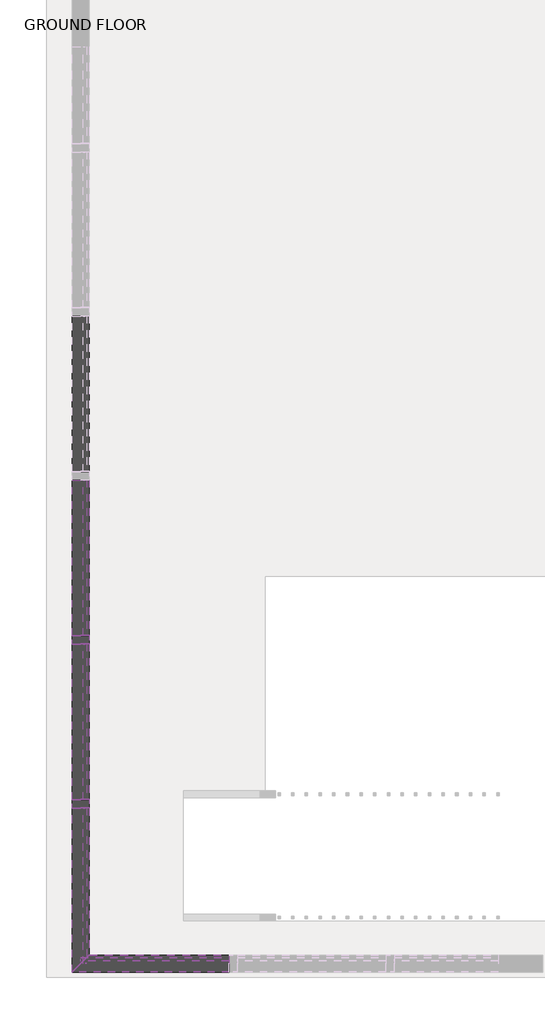
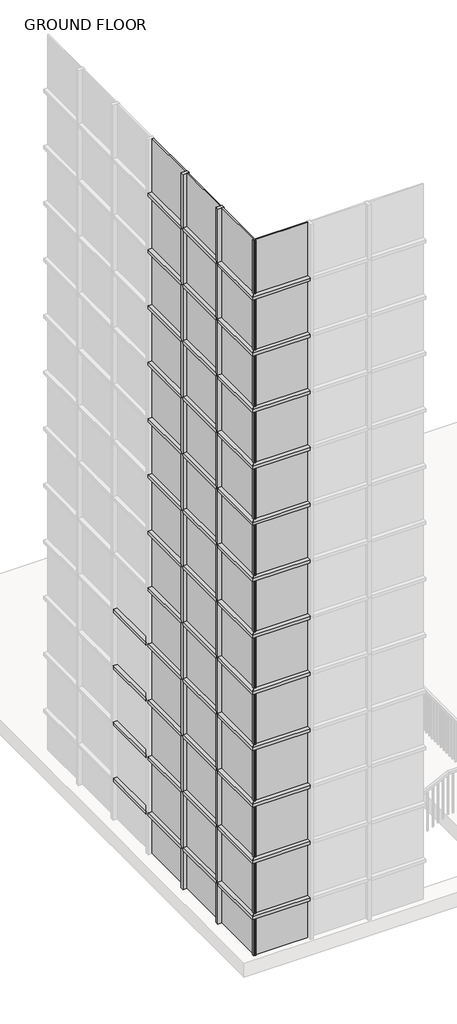
# One storey, part 1 of 16: 78 members, 52 plates.
"""IFC4 building model written with IfcOpenShell, lengths in millimetres."""

from ifc_helpers import new_model, si_unit, origin, place, context, project, spatial, transform, mapped, element, save
from components import member_637f24d3, member_1d29426d, member_b860638c, member_31fee25f, member_49b1bc66, system_panel_glazed_5cba32e5, system_panel_glazed_49652e9e

model = new_model("IFC4")

# Units and contexts
model_context = context("Model", 3, world=origin())
ifc_project = project(units=[si_unit("LENGTHUNIT", "METRE", prefix="MILLI")], contexts=[model_context])

# Site, building, storey
site = spatial("IfcSite", under=ifc_project)
building = spatial("IfcBuilding", under=site)
storey = spatial("IfcBuildingStorey", under=building, Name="GROUND FLOOR", Elevation=0.0)

# Members
placement = place(None, origin())
member_shape = member_637f24d3(model_context)
element("IfcMember", 1, ObjectType="Rectangular Mullion : 2.5\" x 5\" rectangular", at=placement, inside=storey, context=model_context, shape_type="MappedRepresentation", body=[
    mapped(member_shape, transform((-8022.9325224, -5739.2238032, 1168.8884615), x_axis=(0.0, 0.0, 1.0), y_axis=(0.0, -1.0, 0.0), z_axis=(1.0, 0.0, 0.0))),
])
element("IfcMember", 2, ObjectType="Rectangular Mullion : 2.5\" x 5\" rectangular", at=placement, inside=storey, context=model_context, shape_type="MappedRepresentation", body=[
    mapped(member_shape, transform((-8022.9325224, -5739.2238032, 2369.5269231), x_axis=(0.0, 0.0, 1.0), y_axis=(0.0, -1.0, 0.0), z_axis=(1.0, 0.0, 0.0))),
])
element("IfcMember", 3, ObjectType="Rectangular Mullion : 2.5\" x 5\" rectangular", at=placement, inside=storey, context=model_context, shape_type="MappedRepresentation", body=[
    mapped(member_shape, transform((-8022.9325224, -5739.2238032, 3570.1653846), x_axis=(0.0, 0.0, 1.0), y_axis=(0.0, -1.0, 0.0), z_axis=(1.0, 0.0, 0.0))),
])
element("IfcMember", 4, ObjectType="Rectangular Mullion : 2.5\" x 5\" rectangular", at=placement, inside=storey, context=model_context, shape_type="MappedRepresentation", body=[
    mapped(member_shape, transform((-8022.9325224, -5739.2238032, 4770.8038462), x_axis=(0.0, 0.0, 1.0), y_axis=(0.0, -1.0, 0.0), z_axis=(1.0, 0.0, 0.0))),
])
element("IfcMember", 5, ObjectType="Rectangular Mullion : 2.5\" x 5\" rectangular", at=placement, inside=storey, context=model_context, shape_type="MappedRepresentation", body=[
    mapped(member_shape, transform((-8022.9325224, -5739.2238032, 5971.4423077), x_axis=(0.0, 0.0, 1.0), y_axis=(0.0, -1.0, 0.0), z_axis=(1.0, 0.0, 0.0))),
])
element("IfcMember", 6, ObjectType="Rectangular Mullion : 2.5\" x 5\" rectangular", at=placement, inside=storey, context=model_context, shape_type="MappedRepresentation", body=[
    mapped(member_shape, transform((-8022.9325224, -5739.2238032, 7172.0807692), x_axis=(0.0, 0.0, 1.0), y_axis=(0.0, -1.0, 0.0), z_axis=(1.0, 0.0, 0.0))),
])
element("IfcMember", 7, ObjectType="Rectangular Mullion : 2.5\" x 5\" rectangular", at=placement, inside=storey, context=model_context, shape_type="MappedRepresentation", body=[
    mapped(member_shape, transform((-8022.9325224, -5739.2238032, 8372.7192308), x_axis=(0.0, 0.0, 1.0), y_axis=(0.0, -1.0, 0.0), z_axis=(1.0, 0.0, 0.0))),
])
element("IfcMember", 8, ObjectType="Rectangular Mullion : 2.5\" x 5\" rectangular", at=placement, inside=storey, context=model_context, shape_type="MappedRepresentation", body=[
    mapped(member_shape, transform((-8022.9325224, -5739.2238032, 9573.3576923), x_axis=(0.0, 0.0, 1.0), y_axis=(0.0, -1.0, 0.0), z_axis=(1.0, 0.0, 0.0))),
])
element("IfcMember", 9, ObjectType="Rectangular Mullion : 2.5\" x 5\" rectangular", at=placement, inside=storey, context=model_context, shape_type="MappedRepresentation", body=[
    mapped(member_shape, transform((-8022.9325224, -5739.2238032, 10773.9961538), x_axis=(0.0, 0.0, 1.0), y_axis=(0.0, -1.0, 0.0), z_axis=(1.0, 0.0, 0.0))),
])
element("IfcMember", 10, ObjectType="Rectangular Mullion : 2.5\" x 5\" rectangular", at=placement, inside=storey, context=model_context, shape_type="MappedRepresentation", body=[
    mapped(member_shape, transform((-8022.9325224, -5739.2238032, 11974.6346154), x_axis=(0.0, 0.0, 1.0), y_axis=(0.0, -1.0, 0.0), z_axis=(1.0, 0.0, 0.0))),
])
element("IfcMember", 11, ObjectType="Rectangular Mullion : 2.5\" x 5\" rectangular", at=placement, inside=storey, context=model_context, shape_type="MappedRepresentation", body=[
    mapped(member_shape, transform((-8022.9325224, -5739.2238032, 13175.2730769), x_axis=(0.0, 0.0, 1.0), y_axis=(0.0, -1.0, 0.0), z_axis=(1.0, 0.0, 0.0))),
])
element("IfcMember", 12, ObjectType="Rectangular Mullion : 2.5\" x 5\" rectangular", at=placement, inside=storey, context=model_context, shape_type="MappedRepresentation", body=[
    mapped(member_shape, transform((-8022.9325224, -5739.2238032, 14375.9115385), x_axis=(0.0, 0.0, 1.0), y_axis=(0.0, -1.0, 0.0), z_axis=(1.0, 0.0, 0.0))),
])
member_2_shape = member_1d29426d(model_context)
element("IfcMember", 13, ObjectType="Rectangular Mullion : 2.5\" x 5\" rectangular", at=placement, inside=storey, context=model_context, shape_type="MappedRepresentation", body=[
    mapped(member_2_shape, transform((-9124.9017534, -5739.2238032, 1168.8884615), x_axis=(0.0, 0.0, 1.0), y_axis=(-1.0, 0.0, 0.0), z_axis=(0.0, -1.0, 0.0))),
])
element("IfcMember", 14, ObjectType="Rectangular Mullion : 2.5\" x 5\" rectangular", at=placement, inside=storey, context=model_context, shape_type="MappedRepresentation", body=[
    mapped(member_2_shape, transform((-9124.9017534, -5739.2238032, 2369.5269231), x_axis=(0.0, 0.0, 1.0), y_axis=(-1.0, 0.0, 0.0), z_axis=(0.0, -1.0, 0.0))),
])
element("IfcMember", 15, ObjectType="Rectangular Mullion : 2.5\" x 5\" rectangular", at=placement, inside=storey, context=model_context, shape_type="MappedRepresentation", body=[
    mapped(member_2_shape, transform((-9124.9017534, -5739.2238032, 3570.1653846), x_axis=(0.0, 0.0, 1.0), y_axis=(-1.0, 0.0, 0.0), z_axis=(0.0, -1.0, 0.0))),
])
element("IfcMember", 16, ObjectType="Rectangular Mullion : 2.5\" x 5\" rectangular", at=placement, inside=storey, context=model_context, shape_type="MappedRepresentation", body=[
    mapped(member_2_shape, transform((-9124.9017534, -5739.2238032, 4770.8038462), x_axis=(0.0, 0.0, 1.0), y_axis=(-1.0, 0.0, 0.0), z_axis=(0.0, -1.0, 0.0))),
])
element("IfcMember", 17, ObjectType="Rectangular Mullion : 2.5\" x 5\" rectangular", at=placement, inside=storey, context=model_context, shape_type="MappedRepresentation", body=[
    mapped(member_2_shape, transform((-9124.9017534, -5739.2238032, 5971.4423077), x_axis=(0.0, 0.0, 1.0), y_axis=(-1.0, 0.0, 0.0), z_axis=(0.0, -1.0, 0.0))),
])
element("IfcMember", 18, ObjectType="Rectangular Mullion : 2.5\" x 5\" rectangular", at=placement, inside=storey, context=model_context, shape_type="MappedRepresentation", body=[
    mapped(member_2_shape, transform((-9124.9017534, -5739.2238032, 7172.0807692), x_axis=(0.0, 0.0, 1.0), y_axis=(-1.0, 0.0, 0.0), z_axis=(0.0, -1.0, 0.0))),
])
element("IfcMember", 19, ObjectType="Rectangular Mullion : 2.5\" x 5\" rectangular", at=placement, inside=storey, context=model_context, shape_type="MappedRepresentation", body=[
    mapped(member_2_shape, transform((-9124.9017534, -5739.2238032, 8372.7192308), x_axis=(0.0, 0.0, 1.0), y_axis=(-1.0, 0.0, 0.0), z_axis=(0.0, -1.0, 0.0))),
])
element("IfcMember", 20, ObjectType="Rectangular Mullion : 2.5\" x 5\" rectangular", at=placement, inside=storey, context=model_context, shape_type="MappedRepresentation", body=[
    mapped(member_2_shape, transform((-9124.9017534, -5739.2238032, 9573.3576923), x_axis=(0.0, 0.0, 1.0), y_axis=(-1.0, 0.0, 0.0), z_axis=(0.0, -1.0, 0.0))),
])
element("IfcMember", 21, ObjectType="Rectangular Mullion : 2.5\" x 5\" rectangular", at=placement, inside=storey, context=model_context, shape_type="MappedRepresentation", body=[
    mapped(member_2_shape, transform((-9124.9017534, -5739.2238032, 10773.9961538), x_axis=(0.0, 0.0, 1.0), y_axis=(-1.0, 0.0, 0.0), z_axis=(0.0, -1.0, 0.0))),
])
element("IfcMember", 22, ObjectType="Rectangular Mullion : 2.5\" x 5\" rectangular", at=placement, inside=storey, context=model_context, shape_type="MappedRepresentation", body=[
    mapped(member_2_shape, transform((-9124.9017534, -5739.2238032, 11974.6346154), x_axis=(0.0, 0.0, 1.0), y_axis=(-1.0, 0.0, 0.0), z_axis=(0.0, -1.0, 0.0))),
])
element("IfcMember", 23, ObjectType="Rectangular Mullion : 2.5\" x 5\" rectangular", at=placement, inside=storey, context=model_context, shape_type="MappedRepresentation", body=[
    mapped(member_2_shape, transform((-9124.9017534, -5739.2238032, 13175.2730769), x_axis=(0.0, 0.0, 1.0), y_axis=(-1.0, 0.0, 0.0), z_axis=(0.0, -1.0, 0.0))),
])
element("IfcMember", 24, ObjectType="Rectangular Mullion : 2.5\" x 5\" rectangular", at=placement, inside=storey, context=model_context, shape_type="MappedRepresentation", body=[
    mapped(member_2_shape, transform((-9124.9017534, -5739.2238032, 14375.9115385), x_axis=(0.0, 0.0, 1.0), y_axis=(-1.0, 0.0, 0.0), z_axis=(0.0, -1.0, 0.0))),
])
member_3_shape = member_b860638c(model_context)
element("IfcMember", 25, ObjectType="Rectangular Mullion : 2.5\" x 5\" rectangular", at=placement, inside=storey, context=model_context, shape_type="MappedRepresentation", body=[
    mapped(member_3_shape, transform((-9124.9017534, -3336.383803, 0.0), x_axis=(0.0, -1.0, 0.0), y_axis=(-1.0, 0.0, 0.0), z_axis=(0.0, 0.0, -1.0))),
])
element("IfcMember", 26, ObjectType="Rectangular Mullion : 2.5\" x 5\" rectangular", at=placement, inside=storey, context=model_context, shape_type="MappedRepresentation", body=[
    mapped(member_3_shape, transform((-9124.9017534, -4553.678803, 0.0), x_axis=(0.0, -1.0, 0.0), y_axis=(-1.0, 0.0, 0.0), z_axis=(0.0, 0.0, -1.0))),
])
member_4_shape = member_31fee25f(model_context)
element("IfcMember", 27, ObjectType="Rectangular Mullion : 2.5\" x 5\" rectangular", at=placement, inside=storey, context=model_context, shape_type="MappedRepresentation", body=[
    mapped(member_4_shape, transform((-9124.9017534, -3336.383803, 1168.8884615), x_axis=(0.0, -1.0, 0.0), y_axis=(-1.0, 0.0, 0.0), z_axis=(0.0, 0.0, -1.0))),
])
element("IfcMember", 28, ObjectType="Rectangular Mullion : 2.5\" x 5\" rectangular", at=placement, inside=storey, context=model_context, shape_type="MappedRepresentation", body=[
    mapped(member_4_shape, transform((-9124.9017534, -4553.678803, 1168.8884615), x_axis=(0.0, -1.0, 0.0), y_axis=(-1.0, 0.0, 0.0), z_axis=(0.0, 0.0, -1.0))),
])
element("IfcMember", 29, ObjectType="Rectangular Mullion : 2.5\" x 5\" rectangular", at=placement, inside=storey, context=model_context, shape_type="MappedRepresentation", body=[
    mapped(member_4_shape, transform((-9124.9017534, -3336.383803, 2369.5269231), x_axis=(0.0, -1.0, 0.0), y_axis=(-1.0, 0.0, 0.0), z_axis=(0.0, 0.0, -1.0))),
])
element("IfcMember", 30, ObjectType="Rectangular Mullion : 2.5\" x 5\" rectangular", at=placement, inside=storey, context=model_context, shape_type="MappedRepresentation", body=[
    mapped(member_4_shape, transform((-9124.9017534, -4553.678803, 2369.5269231), x_axis=(0.0, -1.0, 0.0), y_axis=(-1.0, 0.0, 0.0), z_axis=(0.0, 0.0, -1.0))),
])
element("IfcMember", 31, ObjectType="Rectangular Mullion : 2.5\" x 5\" rectangular", at=placement, inside=storey, context=model_context, shape_type="MappedRepresentation", body=[
    mapped(member_4_shape, transform((-9124.9017534, -3336.383803, 3570.1653846), x_axis=(0.0, -1.0, 0.0), y_axis=(-1.0, 0.0, 0.0), z_axis=(0.0, 0.0, -1.0))),
])
element("IfcMember", 32, ObjectType="Rectangular Mullion : 2.5\" x 5\" rectangular", at=placement, inside=storey, context=model_context, shape_type="MappedRepresentation", body=[
    mapped(member_4_shape, transform((-9124.9017534, -4553.678803, 3570.1653846), x_axis=(0.0, -1.0, 0.0), y_axis=(-1.0, 0.0, 0.0), z_axis=(0.0, 0.0, -1.0))),
])
element("IfcMember", 33, ObjectType="Rectangular Mullion : 2.5\" x 5\" rectangular", at=placement, inside=storey, context=model_context, shape_type="MappedRepresentation", body=[
    mapped(member_4_shape, transform((-9124.9017534, -3336.383803, 4770.8038462), x_axis=(0.0, -1.0, 0.0), y_axis=(-1.0, 0.0, 0.0), z_axis=(0.0, 0.0, -1.0))),
])
element("IfcMember", 34, ObjectType="Rectangular Mullion : 2.5\" x 5\" rectangular", at=placement, inside=storey, context=model_context, shape_type="MappedRepresentation", body=[
    mapped(member_4_shape, transform((-9124.9017534, -4553.678803, 4770.8038462), x_axis=(0.0, -1.0, 0.0), y_axis=(-1.0, 0.0, 0.0), z_axis=(0.0, 0.0, -1.0))),
])
element("IfcMember", 35, ObjectType="Rectangular Mullion : 2.5\" x 5\" rectangular", at=placement, inside=storey, context=model_context, shape_type="MappedRepresentation", body=[
    mapped(member_4_shape, transform((-9124.9017534, -3336.383803, 5971.4423077), x_axis=(0.0, -1.0, 0.0), y_axis=(-1.0, 0.0, 0.0), z_axis=(0.0, 0.0, -1.0))),
])
element("IfcMember", 36, ObjectType="Rectangular Mullion : 2.5\" x 5\" rectangular", at=placement, inside=storey, context=model_context, shape_type="MappedRepresentation", body=[
    mapped(member_4_shape, transform((-9124.9017534, -4553.678803, 5971.4423077), x_axis=(0.0, -1.0, 0.0), y_axis=(-1.0, 0.0, 0.0), z_axis=(0.0, 0.0, -1.0))),
])
element("IfcMember", 37, ObjectType="Rectangular Mullion : 2.5\" x 5\" rectangular", at=placement, inside=storey, context=model_context, shape_type="MappedRepresentation", body=[
    mapped(member_4_shape, transform((-9124.9017534, -3336.383803, 7172.0807692), x_axis=(0.0, -1.0, 0.0), y_axis=(-1.0, 0.0, 0.0), z_axis=(0.0, 0.0, -1.0))),
])
element("IfcMember", 38, ObjectType="Rectangular Mullion : 2.5\" x 5\" rectangular", at=placement, inside=storey, context=model_context, shape_type="MappedRepresentation", body=[
    mapped(member_4_shape, transform((-9124.9017534, -4553.678803, 7172.0807692), x_axis=(0.0, -1.0, 0.0), y_axis=(-1.0, 0.0, 0.0), z_axis=(0.0, 0.0, -1.0))),
])
element("IfcMember", 39, ObjectType="Rectangular Mullion : 2.5\" x 5\" rectangular", at=placement, inside=storey, context=model_context, shape_type="MappedRepresentation", body=[
    mapped(member_4_shape, transform((-9124.9017534, -3336.383803, 8372.7192308), x_axis=(0.0, -1.0, 0.0), y_axis=(-1.0, 0.0, 0.0), z_axis=(0.0, 0.0, -1.0))),
])
element("IfcMember", 40, ObjectType="Rectangular Mullion : 2.5\" x 5\" rectangular", at=placement, inside=storey, context=model_context, shape_type="MappedRepresentation", body=[
    mapped(member_4_shape, transform((-9124.9017534, -4553.678803, 8372.7192308), x_axis=(0.0, -1.0, 0.0), y_axis=(-1.0, 0.0, 0.0), z_axis=(0.0, 0.0, -1.0))),
])
element("IfcMember", 41, ObjectType="Rectangular Mullion : 2.5\" x 5\" rectangular", at=placement, inside=storey, context=model_context, shape_type="MappedRepresentation", body=[
    mapped(member_4_shape, transform((-9124.9017534, -3336.383803, 9573.3576923), x_axis=(0.0, -1.0, 0.0), y_axis=(-1.0, 0.0, 0.0), z_axis=(0.0, 0.0, -1.0))),
])
element("IfcMember", 42, ObjectType="Rectangular Mullion : 2.5\" x 5\" rectangular", at=placement, inside=storey, context=model_context, shape_type="MappedRepresentation", body=[
    mapped(member_4_shape, transform((-9124.9017534, -4553.678803, 9573.3576923), x_axis=(0.0, -1.0, 0.0), y_axis=(-1.0, 0.0, 0.0), z_axis=(0.0, 0.0, -1.0))),
])
element("IfcMember", 43, ObjectType="Rectangular Mullion : 2.5\" x 5\" rectangular", at=placement, inside=storey, context=model_context, shape_type="MappedRepresentation", body=[
    mapped(member_4_shape, transform((-9124.9017534, -3336.383803, 10773.9961538), x_axis=(0.0, -1.0, 0.0), y_axis=(-1.0, 0.0, 0.0), z_axis=(0.0, 0.0, -1.0))),
])
element("IfcMember", 44, ObjectType="Rectangular Mullion : 2.5\" x 5\" rectangular", at=placement, inside=storey, context=model_context, shape_type="MappedRepresentation", body=[
    mapped(member_4_shape, transform((-9124.9017534, -4553.678803, 10773.9961538), x_axis=(0.0, -1.0, 0.0), y_axis=(-1.0, 0.0, 0.0), z_axis=(0.0, 0.0, -1.0))),
])
element("IfcMember", 45, ObjectType="Rectangular Mullion : 2.5\" x 5\" rectangular", at=placement, inside=storey, context=model_context, shape_type="MappedRepresentation", body=[
    mapped(member_4_shape, transform((-9124.9017534, -3336.383803, 11974.6346154), x_axis=(0.0, -1.0, 0.0), y_axis=(-1.0, 0.0, 0.0), z_axis=(0.0, 0.0, -1.0))),
])
element("IfcMember", 46, ObjectType="Rectangular Mullion : 2.5\" x 5\" rectangular", at=placement, inside=storey, context=model_context, shape_type="MappedRepresentation", body=[
    mapped(member_4_shape, transform((-9124.9017534, -4553.678803, 11974.6346154), x_axis=(0.0, -1.0, 0.0), y_axis=(-1.0, 0.0, 0.0), z_axis=(0.0, 0.0, -1.0))),
])
element("IfcMember", 47, ObjectType="Rectangular Mullion : 2.5\" x 5\" rectangular", at=placement, inside=storey, context=model_context, shape_type="MappedRepresentation", body=[
    mapped(member_4_shape, transform((-9124.9017534, -3336.383803, 13175.2730769), x_axis=(0.0, -1.0, 0.0), y_axis=(-1.0, 0.0, 0.0), z_axis=(0.0, 0.0, -1.0))),
])
element("IfcMember", 48, ObjectType="Rectangular Mullion : 2.5\" x 5\" rectangular", at=placement, inside=storey, context=model_context, shape_type="MappedRepresentation", body=[
    mapped(member_4_shape, transform((-9124.9017534, -4553.678803, 13175.2730769), x_axis=(0.0, -1.0, 0.0), y_axis=(-1.0, 0.0, 0.0), z_axis=(0.0, 0.0, -1.0))),
])
element("IfcMember", 49, ObjectType="Rectangular Mullion : 2.5\" x 5\" rectangular", at=placement, inside=storey, context=model_context, shape_type="MappedRepresentation", body=[
    mapped(member_3_shape, transform((-9124.9017534, -3336.383803, 14375.9115385), x_axis=(0.0, -1.0, 0.0), y_axis=(-1.0, 0.0, 0.0), z_axis=(0.0, 0.0, -1.0))),
])
element("IfcMember", 50, ObjectType="Rectangular Mullion : 2.5\" x 5\" rectangular", at=placement, inside=storey, context=model_context, shape_type="MappedRepresentation", body=[
    mapped(member_3_shape, transform((-9124.9017534, -4553.678803, 14375.9115385), x_axis=(0.0, -1.0, 0.0), y_axis=(-1.0, 0.0, 0.0), z_axis=(0.0, 0.0, -1.0))),
])
member_5_shape = member_49b1bc66(model_context)
element("IfcMember", 51, ObjectType="Rectangular Mullion : 2.5\" x 5\" rectangular", at=placement, inside=storey, context=model_context, shape_type="MappedRepresentation", body=[
    mapped(member_5_shape, transform((-9124.9017534, -2087.3388031, 1168.8884615), x_axis=(0.0, 0.0, 1.0), y_axis=(-1.0, 0.0, 0.0), z_axis=(0.0, -1.0, 0.0))),
])
element("IfcMember", 52, ObjectType="Rectangular Mullion : 2.5\" x 5\" rectangular", at=placement, inside=storey, context=model_context, shape_type="MappedRepresentation", body=[
    mapped(member_5_shape, transform((-9124.9017534, -3304.633803, 1168.8884615), x_axis=(0.0, 0.0, 1.0), y_axis=(-1.0, 0.0, 0.0), z_axis=(0.0, -1.0, 0.0))),
])
element("IfcMember", 53, ObjectType="Rectangular Mullion : 2.5\" x 5\" rectangular", at=placement, inside=storey, context=model_context, shape_type="MappedRepresentation", body=[
    mapped(member_5_shape, transform((-9124.9017534, -4521.928803, 1168.8884615), x_axis=(0.0, 0.0, 1.0), y_axis=(-1.0, 0.0, 0.0), z_axis=(0.0, -1.0, 0.0))),
])
element("IfcMember", 54, ObjectType="Rectangular Mullion : 2.5\" x 5\" rectangular", at=placement, inside=storey, context=model_context, shape_type="MappedRepresentation", body=[
    mapped(member_5_shape, transform((-9124.9017534, -2087.3388031, 2369.5269231), x_axis=(0.0, 0.0, 1.0), y_axis=(-1.0, 0.0, 0.0), z_axis=(0.0, -1.0, 0.0))),
])
element("IfcMember", 55, ObjectType="Rectangular Mullion : 2.5\" x 5\" rectangular", at=placement, inside=storey, context=model_context, shape_type="MappedRepresentation", body=[
    mapped(member_5_shape, transform((-9124.9017534, -3304.633803, 2369.5269231), x_axis=(0.0, 0.0, 1.0), y_axis=(-1.0, 0.0, 0.0), z_axis=(0.0, -1.0, 0.0))),
])
element("IfcMember", 56, ObjectType="Rectangular Mullion : 2.5\" x 5\" rectangular", at=placement, inside=storey, context=model_context, shape_type="MappedRepresentation", body=[
    mapped(member_5_shape, transform((-9124.9017534, -4521.928803, 2369.5269231), x_axis=(0.0, 0.0, 1.0), y_axis=(-1.0, 0.0, 0.0), z_axis=(0.0, -1.0, 0.0))),
])
element("IfcMember", 57, ObjectType="Rectangular Mullion : 2.5\" x 5\" rectangular", at=placement, inside=storey, context=model_context, shape_type="MappedRepresentation", body=[
    mapped(member_5_shape, transform((-9124.9017534, -2087.3388031, 3570.1653846), x_axis=(0.0, 0.0, 1.0), y_axis=(-1.0, 0.0, 0.0), z_axis=(0.0, -1.0, 0.0))),
])
element("IfcMember", 58, ObjectType="Rectangular Mullion : 2.5\" x 5\" rectangular", at=placement, inside=storey, context=model_context, shape_type="MappedRepresentation", body=[
    mapped(member_5_shape, transform((-9124.9017534, -3304.633803, 3570.1653846), x_axis=(0.0, 0.0, 1.0), y_axis=(-1.0, 0.0, 0.0), z_axis=(0.0, -1.0, 0.0))),
])
element("IfcMember", 59, ObjectType="Rectangular Mullion : 2.5\" x 5\" rectangular", at=placement, inside=storey, context=model_context, shape_type="MappedRepresentation", body=[
    mapped(member_5_shape, transform((-9124.9017534, -4521.928803, 3570.1653846), x_axis=(0.0, 0.0, 1.0), y_axis=(-1.0, 0.0, 0.0), z_axis=(0.0, -1.0, 0.0))),
])
element("IfcMember", 60, ObjectType="Rectangular Mullion : 2.5\" x 5\" rectangular", at=placement, inside=storey, context=model_context, shape_type="MappedRepresentation", body=[
    mapped(member_5_shape, transform((-9124.9017534, -2087.3388031, 4770.8038462), x_axis=(0.0, 0.0, 1.0), y_axis=(-1.0, 0.0, 0.0), z_axis=(0.0, -1.0, 0.0))),
])
element("IfcMember", 61, ObjectType="Rectangular Mullion : 2.5\" x 5\" rectangular", at=placement, inside=storey, context=model_context, shape_type="MappedRepresentation", body=[
    mapped(member_5_shape, transform((-9124.9017534, -3304.633803, 4770.8038462), x_axis=(0.0, 0.0, 1.0), y_axis=(-1.0, 0.0, 0.0), z_axis=(0.0, -1.0, 0.0))),
])
element("IfcMember", 62, ObjectType="Rectangular Mullion : 2.5\" x 5\" rectangular", at=placement, inside=storey, context=model_context, shape_type="MappedRepresentation", body=[
    mapped(member_5_shape, transform((-9124.9017534, -4521.928803, 4770.8038462), x_axis=(0.0, 0.0, 1.0), y_axis=(-1.0, 0.0, 0.0), z_axis=(0.0, -1.0, 0.0))),
])
element("IfcMember", 63, ObjectType="Rectangular Mullion : 2.5\" x 5\" rectangular", at=placement, inside=storey, context=model_context, shape_type="MappedRepresentation", body=[
    mapped(member_5_shape, transform((-9124.9017534, -3304.633803, 5971.4423077), x_axis=(0.0, 0.0, 1.0), y_axis=(-1.0, 0.0, 0.0), z_axis=(0.0, -1.0, 0.0))),
])
element("IfcMember", 64, ObjectType="Rectangular Mullion : 2.5\" x 5\" rectangular", at=placement, inside=storey, context=model_context, shape_type="MappedRepresentation", body=[
    mapped(member_5_shape, transform((-9124.9017534, -4521.928803, 5971.4423077), x_axis=(0.0, 0.0, 1.0), y_axis=(-1.0, 0.0, 0.0), z_axis=(0.0, -1.0, 0.0))),
])
element("IfcMember", 65, ObjectType="Rectangular Mullion : 2.5\" x 5\" rectangular", at=placement, inside=storey, context=model_context, shape_type="MappedRepresentation", body=[
    mapped(member_5_shape, transform((-9124.9017534, -3304.633803, 7172.0807692), x_axis=(0.0, 0.0, 1.0), y_axis=(-1.0, 0.0, 0.0), z_axis=(0.0, -1.0, 0.0))),
])
element("IfcMember", 66, ObjectType="Rectangular Mullion : 2.5\" x 5\" rectangular", at=placement, inside=storey, context=model_context, shape_type="MappedRepresentation", body=[
    mapped(member_5_shape, transform((-9124.9017534, -4521.928803, 7172.0807692), x_axis=(0.0, 0.0, 1.0), y_axis=(-1.0, 0.0, 0.0), z_axis=(0.0, -1.0, 0.0))),
])
element("IfcMember", 67, ObjectType="Rectangular Mullion : 2.5\" x 5\" rectangular", at=placement, inside=storey, context=model_context, shape_type="MappedRepresentation", body=[
    mapped(member_5_shape, transform((-9124.9017534, -3304.633803, 8372.7192308), x_axis=(0.0, 0.0, 1.0), y_axis=(-1.0, 0.0, 0.0), z_axis=(0.0, -1.0, 0.0))),
])
element("IfcMember", 68, ObjectType="Rectangular Mullion : 2.5\" x 5\" rectangular", at=placement, inside=storey, context=model_context, shape_type="MappedRepresentation", body=[
    mapped(member_5_shape, transform((-9124.9017534, -4521.928803, 8372.7192308), x_axis=(0.0, 0.0, 1.0), y_axis=(-1.0, 0.0, 0.0), z_axis=(0.0, -1.0, 0.0))),
])
element("IfcMember", 69, ObjectType="Rectangular Mullion : 2.5\" x 5\" rectangular", at=placement, inside=storey, context=model_context, shape_type="MappedRepresentation", body=[
    mapped(member_5_shape, transform((-9124.9017534, -3304.633803, 9573.3576923), x_axis=(0.0, 0.0, 1.0), y_axis=(-1.0, 0.0, 0.0), z_axis=(0.0, -1.0, 0.0))),
])
element("IfcMember", 70, ObjectType="Rectangular Mullion : 2.5\" x 5\" rectangular", at=placement, inside=storey, context=model_context, shape_type="MappedRepresentation", body=[
    mapped(member_5_shape, transform((-9124.9017534, -4521.928803, 9573.3576923), x_axis=(0.0, 0.0, 1.0), y_axis=(-1.0, 0.0, 0.0), z_axis=(0.0, -1.0, 0.0))),
])
element("IfcMember", 71, ObjectType="Rectangular Mullion : 2.5\" x 5\" rectangular", at=placement, inside=storey, context=model_context, shape_type="MappedRepresentation", body=[
    mapped(member_5_shape, transform((-9124.9017534, -3304.633803, 10773.9961538), x_axis=(0.0, 0.0, 1.0), y_axis=(-1.0, 0.0, 0.0), z_axis=(0.0, -1.0, 0.0))),
])
element("IfcMember", 72, ObjectType="Rectangular Mullion : 2.5\" x 5\" rectangular", at=placement, inside=storey, context=model_context, shape_type="MappedRepresentation", body=[
    mapped(member_5_shape, transform((-9124.9017534, -4521.928803, 10773.9961538), x_axis=(0.0, 0.0, 1.0), y_axis=(-1.0, 0.0, 0.0), z_axis=(0.0, -1.0, 0.0))),
])
element("IfcMember", 73, ObjectType="Rectangular Mullion : 2.5\" x 5\" rectangular", at=placement, inside=storey, context=model_context, shape_type="MappedRepresentation", body=[
    mapped(member_5_shape, transform((-9124.9017534, -3304.633803, 11974.6346154), x_axis=(0.0, 0.0, 1.0), y_axis=(-1.0, 0.0, 0.0), z_axis=(0.0, -1.0, 0.0))),
])
element("IfcMember", 74, ObjectType="Rectangular Mullion : 2.5\" x 5\" rectangular", at=placement, inside=storey, context=model_context, shape_type="MappedRepresentation", body=[
    mapped(member_5_shape, transform((-9124.9017534, -4521.928803, 11974.6346154), x_axis=(0.0, 0.0, 1.0), y_axis=(-1.0, 0.0, 0.0), z_axis=(0.0, -1.0, 0.0))),
])
element("IfcMember", 75, ObjectType="Rectangular Mullion : 2.5\" x 5\" rectangular", at=placement, inside=storey, context=model_context, shape_type="MappedRepresentation", body=[
    mapped(member_5_shape, transform((-9124.9017534, -3304.633803, 13175.2730769), x_axis=(0.0, 0.0, 1.0), y_axis=(-1.0, 0.0, 0.0), z_axis=(0.0, -1.0, 0.0))),
])
element("IfcMember", 76, ObjectType="Rectangular Mullion : 2.5\" x 5\" rectangular", at=placement, inside=storey, context=model_context, shape_type="MappedRepresentation", body=[
    mapped(member_5_shape, transform((-9124.9017534, -4521.928803, 13175.2730769), x_axis=(0.0, 0.0, 1.0), y_axis=(-1.0, 0.0, 0.0), z_axis=(0.0, -1.0, 0.0))),
])
element("IfcMember", 77, ObjectType="Rectangular Mullion : 2.5\" x 5\" rectangular", at=placement, inside=storey, context=model_context, shape_type="MappedRepresentation", body=[
    mapped(member_5_shape, transform((-9124.9017534, -3304.633803, 14375.9115385), x_axis=(0.0, 0.0, 1.0), y_axis=(-1.0, 0.0, 0.0), z_axis=(0.0, -1.0, 0.0))),
])
element("IfcMember", 78, ObjectType="Rectangular Mullion : 2.5\" x 5\" rectangular", at=placement, inside=storey, context=model_context, shape_type="MappedRepresentation", body=[
    mapped(member_5_shape, transform((-9124.9017534, -4521.928803, 14375.9115385), x_axis=(0.0, 0.0, 1.0), y_axis=(-1.0, 0.0, 0.0), z_axis=(0.0, -1.0, 0.0))),
])

# Plates
system_panel_glazed_shape = system_panel_glazed_5cba32e5(model_context)
element("IfcPlate", 79, ObjectType="System Panel : Glazed", at=placement, inside=storey, context=model_context, shape_type="MappedRepresentation", body=[
    mapped(system_panel_glazed_shape, transform((-8573.9171379, -5739.2238032, 0.0), x_axis=(1.0, 0.0, 0.0), y_axis=(0.0, 1.0, 0.0), z_axis=(0.0, 0.0, 1.0))),
])
element("IfcPlate", 80, ObjectType="System Panel : Glazed", at=placement, inside=storey, context=model_context, shape_type="MappedRepresentation", body=[
    mapped(system_panel_glazed_shape, transform((-8573.9171379, -5739.2238032, 1200.6384615), x_axis=(1.0, 0.0, 0.0), y_axis=(0.0, 1.0, 0.0), z_axis=(0.0, 0.0, 1.0))),
])
element("IfcPlate", 81, ObjectType="System Panel : Glazed", at=placement, inside=storey, context=model_context, shape_type="MappedRepresentation", body=[
    mapped(system_panel_glazed_shape, transform((-8573.9171379, -5739.2238032, 2401.2769231), x_axis=(1.0, 0.0, 0.0), y_axis=(0.0, 1.0, 0.0), z_axis=(0.0, 0.0, 1.0))),
])
element("IfcPlate", 82, ObjectType="System Panel : Glazed", at=placement, inside=storey, context=model_context, shape_type="MappedRepresentation", body=[
    mapped(system_panel_glazed_shape, transform((-8573.9171379, -5739.2238032, 3601.9153846), x_axis=(1.0, 0.0, 0.0), y_axis=(0.0, 1.0, 0.0), z_axis=(0.0, 0.0, 1.0))),
])
element("IfcPlate", 83, ObjectType="System Panel : Glazed", at=placement, inside=storey, context=model_context, shape_type="MappedRepresentation", body=[
    mapped(system_panel_glazed_shape, transform((-8573.9171379, -5739.2238032, 4802.5538462), x_axis=(1.0, 0.0, 0.0), y_axis=(0.0, 1.0, 0.0), z_axis=(0.0, 0.0, 1.0))),
])
element("IfcPlate", 84, ObjectType="System Panel : Glazed", at=placement, inside=storey, context=model_context, shape_type="MappedRepresentation", body=[
    mapped(system_panel_glazed_shape, transform((-8573.9171379, -5739.2238032, 6003.1923077), x_axis=(1.0, 0.0, 0.0), y_axis=(0.0, 1.0, 0.0), z_axis=(0.0, 0.0, 1.0))),
])
element("IfcPlate", 85, ObjectType="System Panel : Glazed", at=placement, inside=storey, context=model_context, shape_type="MappedRepresentation", body=[
    mapped(system_panel_glazed_shape, transform((-8573.9171379, -5739.2238032, 7203.8307692), x_axis=(1.0, 0.0, 0.0), y_axis=(0.0, 1.0, 0.0), z_axis=(0.0, 0.0, 1.0))),
])
element("IfcPlate", 86, ObjectType="System Panel : Glazed", at=placement, inside=storey, context=model_context, shape_type="MappedRepresentation", body=[
    mapped(system_panel_glazed_shape, transform((-8573.9171379, -5739.2238032, 8404.4692308), x_axis=(1.0, 0.0, 0.0), y_axis=(0.0, 1.0, 0.0), z_axis=(0.0, 0.0, 1.0))),
])
element("IfcPlate", 87, ObjectType="System Panel : Glazed", at=placement, inside=storey, context=model_context, shape_type="MappedRepresentation", body=[
    mapped(system_panel_glazed_shape, transform((-8573.9171379, -5739.2238032, 9605.1076923), x_axis=(1.0, 0.0, 0.0), y_axis=(0.0, 1.0, 0.0), z_axis=(0.0, 0.0, 1.0))),
])
element("IfcPlate", 88, ObjectType="System Panel : Glazed", at=placement, inside=storey, context=model_context, shape_type="MappedRepresentation", body=[
    mapped(system_panel_glazed_shape, transform((-8573.9171379, -5739.2238032, 10805.7461538), x_axis=(1.0, 0.0, 0.0), y_axis=(0.0, 1.0, 0.0), z_axis=(0.0, 0.0, 1.0))),
])
element("IfcPlate", 89, ObjectType="System Panel : Glazed", at=placement, inside=storey, context=model_context, shape_type="MappedRepresentation", body=[
    mapped(system_panel_glazed_shape, transform((-8573.9171379, -5739.2238032, 12006.3846154), x_axis=(1.0, 0.0, 0.0), y_axis=(0.0, 1.0, 0.0), z_axis=(0.0, 0.0, 1.0))),
])
element("IfcPlate", 90, ObjectType="System Panel : Glazed", at=placement, inside=storey, context=model_context, shape_type="MappedRepresentation", body=[
    mapped(system_panel_glazed_shape, transform((-8573.9171379, -5739.2238032, 13207.0230769), x_axis=(1.0, 0.0, 0.0), y_axis=(0.0, 1.0, 0.0), z_axis=(0.0, 0.0, 1.0))),
])
element("IfcPlate", 91, ObjectType="System Panel : Glazed", at=placement, inside=storey, context=model_context, shape_type="MappedRepresentation", body=[
    mapped(system_panel_glazed_shape, transform((-8573.9171379, -5739.2238032, 14407.6615385), x_axis=(1.0, 0.0, 0.0), y_axis=(0.0, 1.0, 0.0), z_axis=(0.0, 0.0, 1.0))),
])
system_panel_glazed_2_shape = system_panel_glazed_49652e9e(model_context)
element("IfcPlate", 92, ObjectType="System Panel : Glazed", at=placement, inside=storey, context=model_context, shape_type="MappedRepresentation", body=[
    mapped(system_panel_glazed_2_shape, transform((-9124.9017534, -2727.7363031, 0.0), x_axis=(0.0, -1.0, 0.0), y_axis=(1.0, 0.0, 0.0), z_axis=(0.0, 0.0, 1.0))),
])
element("IfcPlate", 93, ObjectType="System Panel : Glazed", at=placement, inside=storey, context=model_context, shape_type="MappedRepresentation", body=[
    mapped(system_panel_glazed_2_shape, transform((-9124.9017534, -3945.031303, 0.0), x_axis=(0.0, -1.0, 0.0), y_axis=(1.0, 0.0, 0.0), z_axis=(0.0, 0.0, 1.0))),
])
element("IfcPlate", 94, ObjectType="System Panel : Glazed", at=placement, inside=storey, context=model_context, shape_type="MappedRepresentation", body=[
    mapped(system_panel_glazed_2_shape, transform((-9124.9017534, -5162.3263031, 0.0), x_axis=(0.0, -1.0, 0.0), y_axis=(1.0, 0.0, 0.0), z_axis=(0.0, 0.0, 1.0))),
])
element("IfcPlate", 95, ObjectType="System Panel : Glazed", at=placement, inside=storey, context=model_context, shape_type="MappedRepresentation", body=[
    mapped(system_panel_glazed_2_shape, transform((-9124.9017534, -2727.7363031, 1200.6384615), x_axis=(0.0, -1.0, 0.0), y_axis=(1.0, 0.0, 0.0), z_axis=(0.0, 0.0, 1.0))),
])
element("IfcPlate", 96, ObjectType="System Panel : Glazed", at=placement, inside=storey, context=model_context, shape_type="MappedRepresentation", body=[
    mapped(system_panel_glazed_2_shape, transform((-9124.9017534, -3945.031303, 1200.6384615), x_axis=(0.0, -1.0, 0.0), y_axis=(1.0, 0.0, 0.0), z_axis=(0.0, 0.0, 1.0))),
])
element("IfcPlate", 97, ObjectType="System Panel : Glazed", at=placement, inside=storey, context=model_context, shape_type="MappedRepresentation", body=[
    mapped(system_panel_glazed_2_shape, transform((-9124.9017534, -5162.3263031, 1200.6384615), x_axis=(0.0, -1.0, 0.0), y_axis=(1.0, 0.0, 0.0), z_axis=(0.0, 0.0, 1.0))),
])
element("IfcPlate", 98, ObjectType="System Panel : Glazed", at=placement, inside=storey, context=model_context, shape_type="MappedRepresentation", body=[
    mapped(system_panel_glazed_2_shape, transform((-9124.9017534, -2727.7363031, 2401.2769231), x_axis=(0.0, -1.0, 0.0), y_axis=(1.0, 0.0, 0.0), z_axis=(0.0, 0.0, 1.0))),
])
element("IfcPlate", 99, ObjectType="System Panel : Glazed", at=placement, inside=storey, context=model_context, shape_type="MappedRepresentation", body=[
    mapped(system_panel_glazed_2_shape, transform((-9124.9017534, -3945.031303, 2401.2769231), x_axis=(0.0, -1.0, 0.0), y_axis=(1.0, 0.0, 0.0), z_axis=(0.0, 0.0, 1.0))),
])
element("IfcPlate", 100, ObjectType="System Panel : Glazed", at=placement, inside=storey, context=model_context, shape_type="MappedRepresentation", body=[
    mapped(system_panel_glazed_2_shape, transform((-9124.9017534, -5162.3263031, 2401.2769231), x_axis=(0.0, -1.0, 0.0), y_axis=(1.0, 0.0, 0.0), z_axis=(0.0, 0.0, 1.0))),
])
element("IfcPlate", 101, ObjectType="System Panel : Glazed", at=placement, inside=storey, context=model_context, shape_type="MappedRepresentation", body=[
    mapped(system_panel_glazed_2_shape, transform((-9124.9017534, -2727.7363031, 3601.9153846), x_axis=(0.0, -1.0, 0.0), y_axis=(1.0, 0.0, 0.0), z_axis=(0.0, 0.0, 1.0))),
])
element("IfcPlate", 102, ObjectType="System Panel : Glazed", at=placement, inside=storey, context=model_context, shape_type="MappedRepresentation", body=[
    mapped(system_panel_glazed_2_shape, transform((-9124.9017534, -3945.031303, 3601.9153846), x_axis=(0.0, -1.0, 0.0), y_axis=(1.0, 0.0, 0.0), z_axis=(0.0, 0.0, 1.0))),
])
element("IfcPlate", 103, ObjectType="System Panel : Glazed", at=placement, inside=storey, context=model_context, shape_type="MappedRepresentation", body=[
    mapped(system_panel_glazed_2_shape, transform((-9124.9017534, -5162.3263031, 3601.9153846), x_axis=(0.0, -1.0, 0.0), y_axis=(1.0, 0.0, 0.0), z_axis=(0.0, 0.0, 1.0))),
])
element("IfcPlate", 104, ObjectType="System Panel : Glazed", at=placement, inside=storey, context=model_context, shape_type="MappedRepresentation", body=[
    mapped(system_panel_glazed_2_shape, transform((-9124.9017534, -2727.7363031, 4802.5538462), x_axis=(0.0, -1.0, 0.0), y_axis=(1.0, 0.0, 0.0), z_axis=(0.0, 0.0, 1.0))),
])
element("IfcPlate", 105, ObjectType="System Panel : Glazed", at=placement, inside=storey, context=model_context, shape_type="MappedRepresentation", body=[
    mapped(system_panel_glazed_2_shape, transform((-9124.9017534, -3945.031303, 4802.5538462), x_axis=(0.0, -1.0, 0.0), y_axis=(1.0, 0.0, 0.0), z_axis=(0.0, 0.0, 1.0))),
])
element("IfcPlate", 106, ObjectType="System Panel : Glazed", at=placement, inside=storey, context=model_context, shape_type="MappedRepresentation", body=[
    mapped(system_panel_glazed_2_shape, transform((-9124.9017534, -5162.3263031, 4802.5538462), x_axis=(0.0, -1.0, 0.0), y_axis=(1.0, 0.0, 0.0), z_axis=(0.0, 0.0, 1.0))),
])
element("IfcPlate", 107, ObjectType="System Panel : Glazed", at=placement, inside=storey, context=model_context, shape_type="MappedRepresentation", body=[
    mapped(system_panel_glazed_2_shape, transform((-9124.9017534, -2727.7363031, 6003.1923077), x_axis=(0.0, -1.0, 0.0), y_axis=(1.0, 0.0, 0.0), z_axis=(0.0, 0.0, 1.0))),
])
element("IfcPlate", 108, ObjectType="System Panel : Glazed", at=placement, inside=storey, context=model_context, shape_type="MappedRepresentation", body=[
    mapped(system_panel_glazed_2_shape, transform((-9124.9017534, -3945.031303, 6003.1923077), x_axis=(0.0, -1.0, 0.0), y_axis=(1.0, 0.0, 0.0), z_axis=(0.0, 0.0, 1.0))),
])
element("IfcPlate", 109, ObjectType="System Panel : Glazed", at=placement, inside=storey, context=model_context, shape_type="MappedRepresentation", body=[
    mapped(system_panel_glazed_2_shape, transform((-9124.9017534, -5162.3263031, 6003.1923077), x_axis=(0.0, -1.0, 0.0), y_axis=(1.0, 0.0, 0.0), z_axis=(0.0, 0.0, 1.0))),
])
element("IfcPlate", 110, ObjectType="System Panel : Glazed", at=placement, inside=storey, context=model_context, shape_type="MappedRepresentation", body=[
    mapped(system_panel_glazed_2_shape, transform((-9124.9017534, -2727.7363031, 7203.8307692), x_axis=(0.0, -1.0, 0.0), y_axis=(1.0, 0.0, 0.0), z_axis=(0.0, 0.0, 1.0))),
])
element("IfcPlate", 111, ObjectType="System Panel : Glazed", at=placement, inside=storey, context=model_context, shape_type="MappedRepresentation", body=[
    mapped(system_panel_glazed_2_shape, transform((-9124.9017534, -3945.031303, 7203.8307692), x_axis=(0.0, -1.0, 0.0), y_axis=(1.0, 0.0, 0.0), z_axis=(0.0, 0.0, 1.0))),
])
element("IfcPlate", 112, ObjectType="System Panel : Glazed", at=placement, inside=storey, context=model_context, shape_type="MappedRepresentation", body=[
    mapped(system_panel_glazed_2_shape, transform((-9124.9017534, -5162.3263031, 7203.8307692), x_axis=(0.0, -1.0, 0.0), y_axis=(1.0, 0.0, 0.0), z_axis=(0.0, 0.0, 1.0))),
])
element("IfcPlate", 113, ObjectType="System Panel : Glazed", at=placement, inside=storey, context=model_context, shape_type="MappedRepresentation", body=[
    mapped(system_panel_glazed_2_shape, transform((-9124.9017534, -2727.7363031, 8404.4692308), x_axis=(0.0, -1.0, 0.0), y_axis=(1.0, 0.0, 0.0), z_axis=(0.0, 0.0, 1.0))),
])
element("IfcPlate", 114, ObjectType="System Panel : Glazed", at=placement, inside=storey, context=model_context, shape_type="MappedRepresentation", body=[
    mapped(system_panel_glazed_2_shape, transform((-9124.9017534, -3945.031303, 8404.4692308), x_axis=(0.0, -1.0, 0.0), y_axis=(1.0, 0.0, 0.0), z_axis=(0.0, 0.0, 1.0))),
])
element("IfcPlate", 115, ObjectType="System Panel : Glazed", at=placement, inside=storey, context=model_context, shape_type="MappedRepresentation", body=[
    mapped(system_panel_glazed_2_shape, transform((-9124.9017534, -5162.3263031, 8404.4692308), x_axis=(0.0, -1.0, 0.0), y_axis=(1.0, 0.0, 0.0), z_axis=(0.0, 0.0, 1.0))),
])
element("IfcPlate", 116, ObjectType="System Panel : Glazed", at=placement, inside=storey, context=model_context, shape_type="MappedRepresentation", body=[
    mapped(system_panel_glazed_2_shape, transform((-9124.9017534, -2727.7363031, 9605.1076923), x_axis=(0.0, -1.0, 0.0), y_axis=(1.0, 0.0, 0.0), z_axis=(0.0, 0.0, 1.0))),
])
element("IfcPlate", 117, ObjectType="System Panel : Glazed", at=placement, inside=storey, context=model_context, shape_type="MappedRepresentation", body=[
    mapped(system_panel_glazed_2_shape, transform((-9124.9017534, -3945.031303, 9605.1076923), x_axis=(0.0, -1.0, 0.0), y_axis=(1.0, 0.0, 0.0), z_axis=(0.0, 0.0, 1.0))),
])
element("IfcPlate", 118, ObjectType="System Panel : Glazed", at=placement, inside=storey, context=model_context, shape_type="MappedRepresentation", body=[
    mapped(system_panel_glazed_2_shape, transform((-9124.9017534, -5162.3263031, 9605.1076923), x_axis=(0.0, -1.0, 0.0), y_axis=(1.0, 0.0, 0.0), z_axis=(0.0, 0.0, 1.0))),
])
element("IfcPlate", 119, ObjectType="System Panel : Glazed", at=placement, inside=storey, context=model_context, shape_type="MappedRepresentation", body=[
    mapped(system_panel_glazed_2_shape, transform((-9124.9017534, -2727.7363031, 10805.7461538), x_axis=(0.0, -1.0, 0.0), y_axis=(1.0, 0.0, 0.0), z_axis=(0.0, 0.0, 1.0))),
])
element("IfcPlate", 120, ObjectType="System Panel : Glazed", at=placement, inside=storey, context=model_context, shape_type="MappedRepresentation", body=[
    mapped(system_panel_glazed_2_shape, transform((-9124.9017534, -3945.031303, 10805.7461538), x_axis=(0.0, -1.0, 0.0), y_axis=(1.0, 0.0, 0.0), z_axis=(0.0, 0.0, 1.0))),
])
element("IfcPlate", 121, ObjectType="System Panel : Glazed", at=placement, inside=storey, context=model_context, shape_type="MappedRepresentation", body=[
    mapped(system_panel_glazed_2_shape, transform((-9124.9017534, -5162.3263031, 10805.7461538), x_axis=(0.0, -1.0, 0.0), y_axis=(1.0, 0.0, 0.0), z_axis=(0.0, 0.0, 1.0))),
])
element("IfcPlate", 122, ObjectType="System Panel : Glazed", at=placement, inside=storey, context=model_context, shape_type="MappedRepresentation", body=[
    mapped(system_panel_glazed_2_shape, transform((-9124.9017534, -2727.7363031, 12006.3846154), x_axis=(0.0, -1.0, 0.0), y_axis=(1.0, 0.0, 0.0), z_axis=(0.0, 0.0, 1.0))),
])
element("IfcPlate", 123, ObjectType="System Panel : Glazed", at=placement, inside=storey, context=model_context, shape_type="MappedRepresentation", body=[
    mapped(system_panel_glazed_2_shape, transform((-9124.9017534, -3945.031303, 12006.3846154), x_axis=(0.0, -1.0, 0.0), y_axis=(1.0, 0.0, 0.0), z_axis=(0.0, 0.0, 1.0))),
])
element("IfcPlate", 124, ObjectType="System Panel : Glazed", at=placement, inside=storey, context=model_context, shape_type="MappedRepresentation", body=[
    mapped(system_panel_glazed_2_shape, transform((-9124.9017534, -5162.3263031, 12006.3846154), x_axis=(0.0, -1.0, 0.0), y_axis=(1.0, 0.0, 0.0), z_axis=(0.0, 0.0, 1.0))),
])
element("IfcPlate", 125, ObjectType="System Panel : Glazed", at=placement, inside=storey, context=model_context, shape_type="MappedRepresentation", body=[
    mapped(system_panel_glazed_2_shape, transform((-9124.9017534, -2727.7363031, 13207.0230769), x_axis=(0.0, -1.0, 0.0), y_axis=(1.0, 0.0, 0.0), z_axis=(0.0, 0.0, 1.0))),
])
element("IfcPlate", 126, ObjectType="System Panel : Glazed", at=placement, inside=storey, context=model_context, shape_type="MappedRepresentation", body=[
    mapped(system_panel_glazed_2_shape, transform((-9124.9017534, -3945.031303, 13207.0230769), x_axis=(0.0, -1.0, 0.0), y_axis=(1.0, 0.0, 0.0), z_axis=(0.0, 0.0, 1.0))),
])
element("IfcPlate", 127, ObjectType="System Panel : Glazed", at=placement, inside=storey, context=model_context, shape_type="MappedRepresentation", body=[
    mapped(system_panel_glazed_2_shape, transform((-9124.9017534, -5162.3263031, 13207.0230769), x_axis=(0.0, -1.0, 0.0), y_axis=(1.0, 0.0, 0.0), z_axis=(0.0, 0.0, 1.0))),
])
element("IfcPlate", 128, ObjectType="System Panel : Glazed", at=placement, inside=storey, context=model_context, shape_type="MappedRepresentation", body=[
    mapped(system_panel_glazed_2_shape, transform((-9124.9017534, -2727.7363031, 14407.6615385), x_axis=(0.0, -1.0, 0.0), y_axis=(1.0, 0.0, 0.0), z_axis=(0.0, 0.0, 1.0))),
])
element("IfcPlate", 129, ObjectType="System Panel : Glazed", at=placement, inside=storey, context=model_context, shape_type="MappedRepresentation", body=[
    mapped(system_panel_glazed_2_shape, transform((-9124.9017534, -3945.031303, 14407.6615385), x_axis=(0.0, -1.0, 0.0), y_axis=(1.0, 0.0, 0.0), z_axis=(0.0, 0.0, 1.0))),
])
element("IfcPlate", 130, ObjectType="System Panel : Glazed", at=placement, inside=storey, context=model_context, shape_type="MappedRepresentation", body=[
    mapped(system_panel_glazed_2_shape, transform((-9124.9017534, -5162.3263031, 14407.6615385), x_axis=(0.0, -1.0, 0.0), y_axis=(1.0, 0.0, 0.0), z_axis=(0.0, 0.0, 1.0))),
])

save(model, "model.ifc")

# Revit data of these elements
# Type "Rectangular Mullion : 2.5\" x 5\" rectangular"
#   built-in parameter 1007304 = 0.416667 (stored number, unit not read)
#   built-in parameter 1007301 = 0.104167 (stored number, unit not read)
#   built-in parameter 1007300 = 0.104167 (stored number, unit not read)
# Type "System Panel : Glazed"
#   Construction Type Id = "GSP4R"
#   Analytic Construction = "1/8 in Pilkington single glazing"
#   Visual Light Transmittance = 0.9
#   Solar Heat Gain Coefficient = 0.86
#   Heat Transfer Coefficient (U) = 1.18115 BTU/(h·ft²·°F)
#   Define Thermal Properties by = 1
# Elements 1, 2, 3, 4, 5, 6, 7, 8, 9, 10, 11, 12, 13, 14, 15, 16, 17, 18, 19, 20, 21, 22, 23, 24, 25, 26, 27, 28, 29, 30, 31, 32, 33, 34, 35, 36, 37, 38, 39, 40, 41, 42, 43, 44, 45, 46, 47, 48, 49, 50, 51, 52, 53, 54, 55, 56, 57, 58, 59, 60, 61, 62, 63, 64, 65, 66, 67, 68, 69, 70, 71, 72, 73, 74, 75, 76, 77, 78 (IfcMember, "Rectangular Mullion : 2.5\" x 5\" rectangular")
#   Phase Created = New Construction
#   Materials on its faces: "Aluminum"
# Elements 79, 80, 81, 82, 83, 84, 85, 86, 87, 88, 89, 90, 91, 92, 93, 94, 95, 96, 97, 98, 99, 100, 101, 102, 103, 104, 105, 106, 107, 108, 109, 110, 111, 112, 113, 114, 115, 116, 117, 118, 119, 120, 121, 122, 123, 124, 125, 126, 127, 128, 129, 130 (IfcPlate, "System Panel : Glazed")
#   Phase Created = New Construction
#   Materials on its faces: "Glass"
# Materials
#   "Aluminum": class "Metal", colour RGB 247 247 247, transparency 0, Description = "Aluminum 6061", Cost = 0
#   "Glass": class "Glass", colour RGB 0 128 192, transparency 0.75, Description = "Soda Lime Glass", Cost = 0
